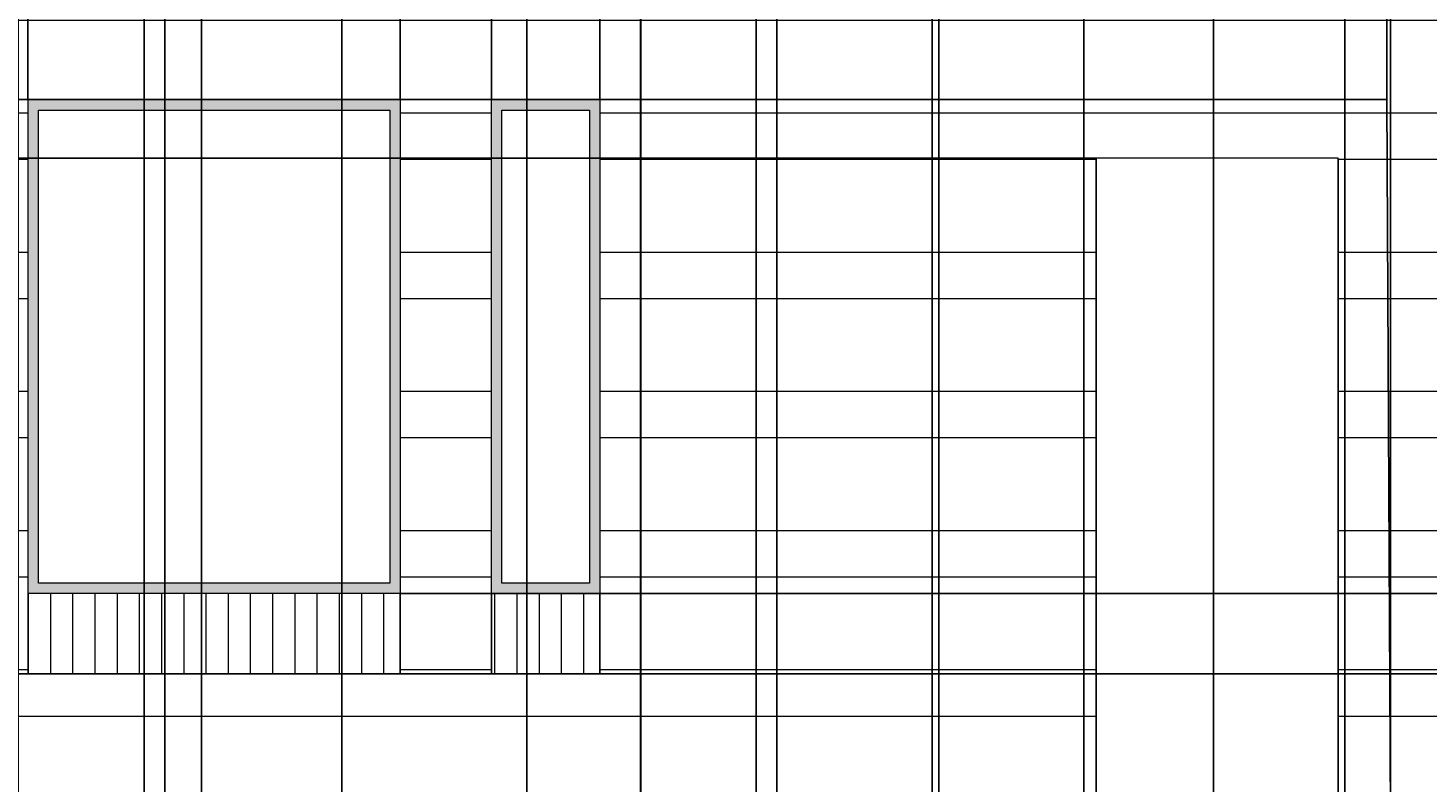
# Model space of a CAD drawing. Units: inches. Extents: x 241 to 943, y 109 to 1396.
# Tile 3 of 34: x 391 to 659, y 253 to 398. Entities that reach past the tile are written whole.
import ezdxf

# ---------------------------------------------------------------- set-up
doc = ezdxf.new("R2010")
doc.units = ezdxf.units.IN
doc.header["$MEASUREMENT"] = 0
for name, color, linetype, lineweight in [('A-ANNO-DIMS', 2, 'Continuous', 18), ('A-ELEV', 7, 'Continuous', 25), ('A-ELEV-SHAD', 9, 'Continuous', 13), ('A-GLAZ', 4, 'Continuous', 18), ('A-GLAZ-PATT', 18, 'Continuous', 13), ('A-WALL-PATT', 8, 'Continuous', 13)]:
    doc.layers.add(name, color=color, linetype=linetype, lineweight=lineweight)
doc.styles.get("Standard").update_dxf_attribs({"font": 'arial.ttf'})
doc.dimstyles.get("Standard").update_dxf_attribs({"dimtxt": 1.4375, "dimasz": 0.18, "dimexe": 0.18, "dimexo": 0.0625, "dimgap": 0.09, "dimtad": 0, "dimtih": 1, "dimtoh": 1, "dimdec": 4, "dimzin": 0, "dimdsep": 46, "dimlunit": 4, "dimtxsty": 'Standard', "dimcen": 0.09, "dimadec": 0, "dimazin": 0, "dimtfac": 1, "dimtdec": 4, "dimtofl": 0, "dimtmove": 0, "dimatfit": 3, "dimfxl": 1, "dimtolj": 1, "dimtzin": 0, "dimarcsym": 0})

# ---------------------------------------------------------------- blocks, each defined once
blk = doc.blocks.new('*D7')
at = {"layer": 'A-ANNO-DIMS', "color": 0, "lineweight": -2, "transparency": 16777216}
for p, q in [((508.24, 1336.12), (244.31, 1336.12)), ((244.49, 1335.94), (244.49, 753.25)), ((244.49, 168.92), (244.49, 751.6)), ((303.17, 168.74), (244.31, 168.74))]:
    blk.add_line(p, q, dxfattribs=at)
at = {"layer": 'A-ANNO-DIMS', "color": 0, "transparency": 16777216}
for points in [[(244.46, 1335.94), (244.52, 1335.94), (244.49, 1336.12)], [(244.46, 168.92), (244.52, 168.92), (244.49, 168.74)]]:
    blk.add_solid(points, dxfattribs=at)
at = {"layer": 'Defpoints', "color": 0, "transparency": 16777216}
for p in [(244.49, 1336.12), (508.31, 1336.12), (303.24, 168.74)]:
    blk.add_point(p, dxfattribs=at)
at = {"layer": 'A-ANNO-DIMS', "color": 0, "transparency": 16777216, "insert": (244.49, 752.43), "char_height": 1.438, "attachment_point": 5}
blk.add_mtext('\\A1;1167.4', dxfattribs=at)
blk = doc.blocks.new('*D9')
at = {"layer": 'A-ANNO-DIMS', "color": 0, "lineweight": -2, "transparency": 16777216}
for p, q in [((390.89, 384.24), (390.89, 1395.05)), ((391.07, 1394.87), (424.13, 1394.87)), ((461.93, 1394.87), (428.87, 1394.87)), ((462.11, 384.24), (462.11, 1395.05))]:
    blk.add_line(p, q, dxfattribs=at)
at = {"layer": 'A-ANNO-DIMS', "color": 0, "transparency": 16777216}
for points in [[(391.07, 1394.9), (391.07, 1394.84), (390.89, 1394.87)], [(461.93, 1394.9), (461.93, 1394.84), (462.11, 1394.87)]]:
    blk.add_solid(points, dxfattribs=at)
at = {"layer": 'Defpoints', "color": 0, "transparency": 16777216}
for p in [(462.11, 1394.87), (390.89, 384.18), (462.11, 384.18)]:
    blk.add_point(p, dxfattribs=at)
at = {"layer": 'A-ANNO-DIMS', "color": 0, "transparency": 16777216, "insert": (426.5, 1394.87), "char_height": 1.438, "attachment_point": 5}
blk.add_mtext('\\A1;71.21', dxfattribs=at)
blk = doc.blocks.new('*D10')
at = {"layer": 'A-ANNO-DIMS', "color": 0, "lineweight": -2, "transparency": 16777216}
for p, q in [((462.11, 384.24), (462.11, 1395.05)), ((462.29, 1394.87), (468.4, 1394.87)), ((479.42, 1394.87), (473.3, 1394.87)), ((479.6, 384.24), (479.6, 1395.05))]:
    blk.add_line(p, q, dxfattribs=at)
at = {"layer": 'A-ANNO-DIMS', "color": 0, "transparency": 16777216}
for points in [[(462.29, 1394.9), (462.29, 1394.84), (462.11, 1394.87)], [(479.42, 1394.9), (479.42, 1394.84), (479.6, 1394.87)]]:
    blk.add_solid(points, dxfattribs=at)
at = {"layer": 'Defpoints', "color": 0, "transparency": 16777216}
for p in [(479.6, 1394.87), (462.11, 384.18), (479.6, 384.18)]:
    blk.add_point(p, dxfattribs=at)
at = {"layer": 'A-ANNO-DIMS', "color": 0, "transparency": 16777216, "insert": (470.85, 1394.87), "char_height": 1.438, "attachment_point": 5}
blk.add_mtext('\\A1;17.49', dxfattribs=at)
blk = doc.blocks.new('*D11')
at = {"layer": 'A-ANNO-DIMS', "color": 0, "lineweight": -2, "transparency": 16777216}
for p, q in [((500.33, 384.24), (500.33, 1395.05)), ((500.51, 1394.87), (513.31, 1394.87)), ((530.05, 1394.87), (517.25, 1394.87)), ((530.23, 384.24), (530.23, 1395.05))]:
    blk.add_line(p, q, dxfattribs=at)
at = {"layer": 'A-ANNO-DIMS', "color": 0, "transparency": 16777216}
for points in [[(500.51, 1394.9), (500.51, 1394.84), (500.33, 1394.87)], [(530.05, 1394.9), (530.05, 1394.84), (530.23, 1394.87)]]:
    blk.add_solid(points, dxfattribs=at)
at = {"layer": 'Defpoints', "color": 0, "transparency": 16777216}
for p in [(530.23, 1394.87), (500.33, 384.18), (530.23, 384.18)]:
    blk.add_point(p, dxfattribs=at)
at = {"layer": 'A-ANNO-DIMS', "color": 0, "transparency": 16777216, "insert": (515.28, 1394.87), "char_height": 1.438, "attachment_point": 5}
blk.add_mtext('\\A1;29.9', dxfattribs=at)
blk = doc.blocks.new('*D12')
at = {"layer": 'A-ANNO-DIMS', "color": 0, "lineweight": -2, "transparency": 16777216}
for p, q in [((530.23, 384.24), (530.23, 1395.05)), ((530.41, 1394.87), (587.56, 1394.87)), ((650.73, 1394.87), (593.58, 1394.87)), ((650.91, 384.24), (650.91, 1395.05))]:
    blk.add_line(p, q, dxfattribs=at)
at = {"layer": 'A-ANNO-DIMS', "color": 0, "transparency": 16777216}
for points in [[(530.41, 1394.9), (530.41, 1394.84), (530.23, 1394.87)], [(650.73, 1394.9), (650.73, 1394.84), (650.91, 1394.87)]]:
    blk.add_solid(points, dxfattribs=at)
at = {"layer": 'Defpoints', "color": 0, "transparency": 16777216}
for p in [(650.91, 1394.87), (530.23, 384.18), (650.91, 384.18)]:
    blk.add_point(p, dxfattribs=at)
at = {"layer": 'A-ANNO-DIMS', "color": 0, "transparency": 16777216, "insert": (590.57, 1394.87), "char_height": 1.438, "attachment_point": 5}
blk.add_mtext('\\A1;120.68', dxfattribs=at)
blk = doc.blocks.new('*D13')
at = {"layer": 'A-ANNO-DIMS', "color": 0, "lineweight": -2, "transparency": 16777216}
for p, q in [((650.91, 384.24), (650.91, 1395.05)), ((651.09, 1394.87), (656.14, 1394.87)), ((667.21, 1394.87), (662.16, 1394.87)), ((667.39, 290.06), (667.39, 1395.05))]:
    blk.add_line(p, q, dxfattribs=at)
at = {"layer": 'A-ANNO-DIMS', "color": 0, "transparency": 16777216}
for points in [[(651.09, 1394.9), (651.09, 1394.84), (650.91, 1394.87)], [(667.21, 1394.9), (667.21, 1394.84), (667.39, 1394.87)]]:
    blk.add_solid(points, dxfattribs=at)
at = {"layer": 'Defpoints', "color": 0, "transparency": 16777216}
for p in [(667.39, 1394.87), (650.91, 384.18), (667.39, 290)]:
    blk.add_point(p, dxfattribs=at)
at = {"layer": 'A-ANNO-DIMS', "color": 0, "transparency": 16777216, "insert": (659.15, 1394.87), "char_height": 1.438, "attachment_point": 5}
blk.add_mtext('\\A1;16.486', dxfattribs=at)
blk = doc.blocks.new('*D16')
at = {"layer": 'A-ANNO-DIMS', "color": 0, "lineweight": -2, "transparency": 16777216}
for p, q in [((595.31, 372.88), (595.31, 109.81)), ((641.62, 372.88), (641.62, 109.81)), ((595.49, 109.99), (616.06, 109.99)), ((641.44, 109.99), (620.87, 109.99))]:
    blk.add_line(p, q, dxfattribs=at)
at = {"layer": 'A-ANNO-DIMS', "color": 0, "transparency": 16777216}
for points in [[(595.49, 110.02), (595.49, 109.96), (595.31, 109.99)], [(641.44, 110.02), (641.44, 109.96), (641.62, 109.99)]]:
    blk.add_solid(points, dxfattribs=at)
at = {"layer": 'Defpoints', "color": 0, "transparency": 16777216}
for p in [(595.31, 372.94), (641.62, 372.94), (641.62, 109.99)]:
    blk.add_point(p, dxfattribs=at)
at = {"layer": 'A-ANNO-DIMS', "color": 0, "transparency": 16777216, "insert": (618.47, 109.99), "char_height": 1.438, "attachment_point": 5}
blk.add_mtext('\\A1;46.31', dxfattribs=at)
blk = doc.blocks.new('*D29')
at = {"layer": 'A-ANNO-DIMS', "color": 0, "lineweight": -2, "transparency": 16777216}
for p, q in [((462.17, 289.69), (940.6, 289.69)), ((940.42, 289.51), (940.42, 282.85)), ((940.42, 274.53), (940.42, 281.2)), ((462.17, 274.35), (940.6, 274.35))]:
    blk.add_line(p, q, dxfattribs=at)
at = {"layer": 'A-ANNO-DIMS', "color": 0, "transparency": 16777216}
for points in [[(940.39, 289.51), (940.45, 289.51), (940.42, 289.69)], [(940.39, 274.53), (940.45, 274.53), (940.42, 274.35)]]:
    blk.add_solid(points, dxfattribs=at)
at = {"layer": 'Defpoints', "color": 0, "transparency": 16777216}
for p in [(462.11, 289.69), (940.42, 289.69), (462.11, 274.35)]:
    blk.add_point(p, dxfattribs=at)
at = {"layer": 'A-ANNO-DIMS', "color": 0, "transparency": 16777216, "insert": (940.42, 282.02), "char_height": 1.438, "attachment_point": 5}
blk.add_mtext('\\A1;15.343', dxfattribs=at)
blk = doc.blocks.new('*D41')
at = {"layer": 'A-ANNO-DIMS', "color": 0, "lineweight": -2, "transparency": 16777216}
for p, q in [((820.77, 400.83), (244.31, 400.83)), ((244.49, 400.65), (244.49, 317.65)), ((244.49, 233.01), (244.49, 316.01)), ((820.77, 232.83), (244.31, 232.83))]:
    blk.add_line(p, q, dxfattribs=at)
at = {"layer": 'A-ANNO-DIMS', "color": 0, "transparency": 16777216}
for points in [[(244.46, 400.65), (244.52, 400.65), (244.49, 400.83)], [(244.46, 233.01), (244.52, 233.01), (244.49, 232.83)]]:
    blk.add_solid(points, dxfattribs=at)
at = {"layer": 'Defpoints', "color": 0, "transparency": 16777216}
for p in [(244.49, 400.83), (820.84, 400.83), (820.84, 232.83)]:
    blk.add_point(p, dxfattribs=at)
at = {"layer": 'A-ANNO-DIMS', "color": 0, "transparency": 16777216, "insert": (244.49, 316.83), "char_height": 1.438, "attachment_point": 5}
blk.add_mtext('\\A1;168', dxfattribs=at)
blk = doc.blocks.new('*D51')
at = {"layer": 'A-ANNO-DIMS', "color": 0, "lineweight": -2, "transparency": 16777216}
for p, q in [((595.25, 372.94), (244.31, 372.94)), ((244.49, 372.76), (244.49, 310.39)), ((244.49, 246.38), (244.49, 308.74)), ((595.25, 246.2), (244.31, 246.2))]:
    blk.add_line(p, q, dxfattribs=at)
at = {"layer": 'A-ANNO-DIMS', "color": 0, "transparency": 16777216}
for points in [[(244.46, 372.76), (244.52, 372.76), (244.49, 372.94)], [(244.46, 246.38), (244.52, 246.38), (244.49, 246.2)]]:
    blk.add_solid(points, dxfattribs=at)
at = {"layer": 'Defpoints', "color": 0, "transparency": 16777216}
for p in [(244.49, 372.94), (595.31, 372.94), (595.31, 246.2)]:
    blk.add_point(p, dxfattribs=at)
at = {"layer": 'A-ANNO-DIMS', "color": 0, "transparency": 16777216, "insert": (244.49, 309.57), "char_height": 1.438, "attachment_point": 5}
blk.add_mtext('\\A1;126.74', dxfattribs=at)
blk = doc.blocks.new('*D52')
at = {"layer": 'A-ANNO-DIMS', "color": 0, "lineweight": -2, "transparency": 16777216}
for p, q in [((530.17, 384.18), (244.31, 384.18)), ((244.49, 384), (244.49, 315.83)), ((244.49, 246.02), (244.49, 314.18)), ((530.17, 245.84), (244.31, 245.84))]:
    blk.add_line(p, q, dxfattribs=at)
at = {"layer": 'A-ANNO-DIMS', "color": 0, "transparency": 16777216}
for points in [[(244.46, 384), (244.52, 384), (244.49, 384.18)], [(244.46, 246.02), (244.52, 246.02), (244.49, 245.84)]]:
    blk.add_solid(points, dxfattribs=at)
at = {"layer": 'Defpoints', "color": 0, "transparency": 16777216}
for p in [(244.49, 384.18), (530.23, 384.18), (530.23, 245.84)]:
    blk.add_point(p, dxfattribs=at)
at = {"layer": 'A-ANNO-DIMS', "color": 0, "transparency": 16777216, "insert": (244.49, 315.01), "char_height": 1.438, "attachment_point": 5}
blk.add_mtext('\\A1;138.34', dxfattribs=at)
blk = doc.blocks.new('*D79')
at = {"layer": 'A-ANNO-DIMS', "color": 0, "lineweight": -2, "transparency": 16777216}
for p, q in [((479.6, 384.24), (479.6, 1395.05)), ((479.78, 1394.87), (486.88, 1394.87)), ((500.15, 1394.87), (493.05, 1394.87)), ((500.33, 384.24), (500.33, 1395.05))]:
    blk.add_line(p, q, dxfattribs=at)
at = {"layer": 'A-ANNO-DIMS', "color": 0, "transparency": 16777216}
for points in [[(479.78, 1394.9), (479.78, 1394.84), (479.6, 1394.87)], [(500.15, 1394.9), (500.15, 1394.84), (500.33, 1394.87)]]:
    blk.add_solid(points, dxfattribs=at)
at = {"layer": 'Defpoints', "color": 0, "transparency": 16777216}
for p in [(500.33, 1394.87), (479.6, 384.18), (500.33, 384.18)]:
    blk.add_point(p, dxfattribs=at)
at = {"layer": 'A-ANNO-DIMS', "color": 0, "transparency": 16777216, "insert": (489.96, 1394.87), "char_height": 1.438, "attachment_point": 5}
blk.add_mtext('\\A1;20.736', dxfattribs=at)
blk = doc.blocks.new('*D80')
at = {"layer": 'A-ANNO-DIMS', "color": 0, "lineweight": -2, "transparency": 16777216}
for p, q in [((530.23, 384.12), (530.23, 109.81)), ((595.31, 372.88), (595.31, 109.81)), ((530.41, 109.99), (560.25, 109.99)), ((595.13, 109.99), (565.29, 109.99))]:
    blk.add_line(p, q, dxfattribs=at)
at = {"layer": 'A-ANNO-DIMS', "color": 0, "transparency": 16777216}
for points in [[(530.41, 110.02), (530.41, 109.96), (530.23, 109.99)], [(595.13, 110.02), (595.13, 109.96), (595.31, 109.99)]]:
    blk.add_solid(points, dxfattribs=at)
at = {"layer": 'Defpoints', "color": 0, "transparency": 16777216}
for p in [(530.23, 384.18), (595.31, 372.94), (595.31, 109.99)]:
    blk.add_point(p, dxfattribs=at)
at = {"layer": 'A-ANNO-DIMS', "color": 0, "transparency": 16777216, "insert": (562.77, 109.99), "char_height": 1.438, "attachment_point": 5}
blk.add_mtext('\\A1;65.08', dxfattribs=at)
blk = doc.blocks.new('*D81')
at = {"layer": 'A-ANNO-DIMS', "color": 0, "lineweight": -2, "transparency": 16777216}
for p, q in [((462.04, 274.35), (244.31, 274.35)), ((244.49, 274.17), (244.49, 260.92)), ((244.49, 246.02), (244.49, 259.27)), ((530.17, 245.84), (244.31, 245.84))]:
    blk.add_line(p, q, dxfattribs=at)
at = {"layer": 'A-ANNO-DIMS', "color": 0, "transparency": 16777216}
for points in [[(244.46, 274.17), (244.52, 274.17), (244.49, 274.35)], [(244.46, 246.02), (244.52, 246.02), (244.49, 245.84)]]:
    blk.add_solid(points, dxfattribs=at)
at = {"layer": 'Defpoints', "color": 0, "transparency": 16777216}
for p in [(244.49, 274.35), (462.11, 274.35), (530.23, 245.84)]:
    blk.add_point(p, dxfattribs=at)
at = {"layer": 'A-ANNO-DIMS', "color": 0, "transparency": 16777216, "insert": (244.49, 260.09), "char_height": 1.438, "attachment_point": 5}
blk.add_mtext('\\A1;28.51', dxfattribs=at)
blk = doc.blocks.new('*D99')
at = {"layer": 'A-ANNO-DIMS', "color": 0, "lineweight": -2, "transparency": 16777216}
for p, q in [((417.09, 181.71), (417.09, 1395.05)), ((417.27, 1394.87), (539.16, 1394.87)), ((667.21, 1394.87), (545.33, 1394.87)), ((667.39, 214.58), (667.39, 1395.05))]:
    blk.add_line(p, q, dxfattribs=at)
at = {"layer": 'A-ANNO-DIMS', "color": 0, "transparency": 16777216}
for points in [[(417.27, 1394.9), (417.27, 1394.84), (417.09, 1394.87)], [(667.21, 1394.9), (667.21, 1394.84), (667.39, 1394.87)]]:
    blk.add_solid(points, dxfattribs=at)
at = {"layer": 'Defpoints', "color": 0, "transparency": 16777216}
for p in [(667.39, 1394.87), (667.39, 214.52), (417.09, 181.65)]:
    blk.add_point(p, dxfattribs=at)
at = {"layer": 'A-ANNO-DIMS', "color": 0, "transparency": 16777216, "insert": (542.24, 1394.87), "char_height": 1.438, "attachment_point": 5}
blk.add_mtext('\\A1;250.30', dxfattribs=at)
blk = doc.blocks.new('*D119')
at = {"layer": 'A-ANNO-DIMS', "color": 0, "lineweight": -2, "transparency": 16777216}
for p, q in [((617.76, 734.79), (617.76, 109.81)), ((642.92, 734.79), (642.92, 109.81)), ((617.94, 109.99), (627.81, 109.99)), ((642.74, 109.99), (632.87, 109.99))]:
    blk.add_line(p, q, dxfattribs=at)
at = {"layer": 'A-ANNO-DIMS', "color": 0, "transparency": 16777216}
for points in [[(617.94, 110.02), (617.94, 109.96), (617.76, 109.99)], [(642.74, 110.02), (642.74, 109.96), (642.92, 109.99)]]:
    blk.add_solid(points, dxfattribs=at)
at = {"layer": 'Defpoints', "color": 0, "transparency": 16777216}
for p in [(617.76, 734.85), (642.92, 734.85), (642.92, 109.99)]:
    blk.add_point(p, dxfattribs=at)
at = {"layer": 'A-ANNO-DIMS', "color": 0, "transparency": 16777216, "insert": (630.34, 109.99), "char_height": 1.438, "attachment_point": 5}
blk.add_mtext('\\A1;25.16', dxfattribs=at)
blk = doc.blocks.new('*D120')
at = {"layer": 'A-ANNO-DIMS', "color": 0, "lineweight": -2, "transparency": 16777216}
for p, q in [((642.92, 734.79), (642.92, 109.81)), ((678.27, 734.79), (678.27, 109.81)), ((643.1, 109.99), (658.07, 109.99)), ((678.09, 109.99), (663.11, 109.99))]:
    blk.add_line(p, q, dxfattribs=at)
at = {"layer": 'A-ANNO-DIMS', "color": 0, "transparency": 16777216}
for points in [[(643.1, 110.02), (643.1, 109.96), (642.92, 109.99)], [(678.09, 110.02), (678.09, 109.96), (678.27, 109.99)]]:
    blk.add_solid(points, dxfattribs=at)
at = {"layer": 'Defpoints', "color": 0, "transparency": 16777216}
for p in [(642.92, 734.85), (678.27, 734.85), (678.27, 109.99)]:
    blk.add_point(p, dxfattribs=at)
at = {"layer": 'A-ANNO-DIMS', "color": 0, "transparency": 16777216, "insert": (660.59, 109.99), "char_height": 1.438, "attachment_point": 5}
blk.add_mtext('\\A1;35.35', dxfattribs=at)
blk = doc.blocks.new('*D126')
at = {"layer": 'A-ANNO-DIMS', "color": 0, "lineweight": -2, "transparency": 16777216}
for p, q in [((450.93, 651.27), (450.93, 109.81)), ((424.11, 628.34), (424.11, 109.81)), ((424.29, 109.99), (434.43, 109.99)), ((450.75, 109.99), (440.6, 109.99))]:
    blk.add_line(p, q, dxfattribs=at)
at = {"layer": 'A-ANNO-DIMS', "color": 0, "transparency": 16777216}
for points in [[(424.29, 110.02), (424.29, 109.96), (424.11, 109.99)], [(450.75, 110.02), (450.75, 109.96), (450.93, 109.99)]]:
    blk.add_solid(points, dxfattribs=at)
at = {"layer": 'Defpoints', "color": 0, "transparency": 16777216}
for p in [(450.93, 651.34), (424.11, 628.4), (450.93, 109.99)]:
    blk.add_point(p, dxfattribs=at)
at = {"layer": 'A-ANNO-DIMS', "color": 0, "transparency": 16777216, "insert": (437.52, 109.99), "char_height": 1.438, "attachment_point": 5}
blk.add_mtext('\\A1;26.817', dxfattribs=at)
blk = doc.blocks.new('*D127')
at = {"layer": 'A-ANNO-DIMS', "color": 0, "lineweight": -2, "transparency": 16777216}
for p, q in [((450.93, 651.27), (450.93, 109.81)), ((508.19, 630.34), (508.19, 109.81)), ((451.11, 109.99), (477.04, 109.99)), ((508.01, 109.99), (482.07, 109.99))]:
    blk.add_line(p, q, dxfattribs=at)
at = {"layer": 'A-ANNO-DIMS', "color": 0, "transparency": 16777216}
for points in [[(451.11, 110.02), (451.11, 109.96), (450.93, 109.99)], [(508.01, 110.02), (508.01, 109.96), (508.19, 109.99)]]:
    blk.add_solid(points, dxfattribs=at)
at = {"layer": 'Defpoints', "color": 0, "transparency": 16777216}
for p in [(450.93, 651.34), (508.19, 630.4), (508.19, 109.99)]:
    blk.add_point(p, dxfattribs=at)
at = {"layer": 'A-ANNO-DIMS', "color": 0, "transparency": 16777216, "insert": (479.56, 109.99), "char_height": 1.438, "attachment_point": 5}
blk.add_mtext('\\A1;57.26', dxfattribs=at)
blk = doc.blocks.new('*D128')
at = {"layer": 'A-ANNO-DIMS', "color": 0, "lineweight": -2, "transparency": 16777216}
for p, q in [((534.18, 651.27), (534.18, 109.81)), ((508.19, 630.34), (508.19, 109.81)), ((508.37, 109.99), (518.1, 109.99)), ((534, 109.99), (524.27, 109.99))]:
    blk.add_line(p, q, dxfattribs=at)
at = {"layer": 'A-ANNO-DIMS', "color": 0, "transparency": 16777216}
for points in [[(508.37, 110.02), (508.37, 109.96), (508.19, 109.99)], [(534, 110.02), (534, 109.96), (534.18, 109.99)]]:
    blk.add_solid(points, dxfattribs=at)
at = {"layer": 'Defpoints', "color": 0, "transparency": 16777216}
for p in [(534.18, 651.34), (508.19, 630.4), (534.18, 109.99)]:
    blk.add_point(p, dxfattribs=at)
at = {"layer": 'A-ANNO-DIMS', "color": 0, "transparency": 16777216, "insert": (521.18, 109.99), "char_height": 1.438, "attachment_point": 5}
blk.add_mtext('\\A1;25.987', dxfattribs=at)
blk = doc.blocks.new('*D129')
at = {"layer": 'A-ANNO-DIMS', "color": 0, "lineweight": -2, "transparency": 16777216}
for p, q in [((534.18, 651.27), (534.18, 109.81)), ((563.93, 651.27), (563.93, 109.81)), ((534.36, 109.99), (546.52, 109.99)), ((563.75, 109.99), (551.59, 109.99))]:
    blk.add_line(p, q, dxfattribs=at)
at = {"layer": 'A-ANNO-DIMS', "color": 0, "transparency": 16777216}
for points in [[(534.36, 110.02), (534.36, 109.96), (534.18, 109.99)], [(563.75, 110.02), (563.75, 109.96), (563.93, 109.99)]]:
    blk.add_solid(points, dxfattribs=at)
at = {"layer": 'Defpoints', "color": 0, "transparency": 16777216}
for p in [(534.18, 651.34), (563.93, 651.34), (563.93, 109.99)]:
    blk.add_point(p, dxfattribs=at)
at = {"layer": 'A-ANNO-DIMS', "color": 0, "transparency": 16777216, "insert": (549.05, 109.99), "char_height": 1.438, "attachment_point": 5}
blk.add_mtext('\\A1;29.75', dxfattribs=at)
blk = doc.blocks.new('*D130')
at = {"layer": 'A-ANNO-DIMS', "color": 0, "lineweight": -2, "transparency": 16777216}
for p, q in [((563.93, 651.27), (563.93, 109.81)), ((592.95, 628.34), (592.95, 109.81)), ((564.11, 109.99), (575.35, 109.99)), ((592.77, 109.99), (581.53, 109.99))]:
    blk.add_line(p, q, dxfattribs=at)
at = {"layer": 'A-ANNO-DIMS', "color": 0, "transparency": 16777216}
for points in [[(564.11, 110.02), (564.11, 109.96), (563.93, 109.99)], [(592.77, 110.02), (592.77, 109.96), (592.95, 109.99)]]:
    blk.add_solid(points, dxfattribs=at)
at = {"layer": 'Defpoints', "color": 0, "transparency": 16777216}
for p in [(563.93, 651.34), (592.95, 628.4), (592.95, 109.99)]:
    blk.add_point(p, dxfattribs=at)
at = {"layer": 'A-ANNO-DIMS', "color": 0, "transparency": 16777216, "insert": (578.44, 109.99), "char_height": 1.438, "attachment_point": 5}
blk.add_mtext('\\A1;29.025', dxfattribs=at)
blk = doc.blocks.new('*D132')
at = {"layer": 'A-ANNO-DIMS', "color": 0, "lineweight": -2, "transparency": 16777216}
for p, q in [((676.87, 628.34), (676.87, 109.81)), ((617.76, 626.34), (617.76, 109.81)), ((617.94, 109.99), (644.94, 109.99)), ((676.69, 109.99), (649.69, 109.99))]:
    blk.add_line(p, q, dxfattribs=at)
at = {"layer": 'A-ANNO-DIMS', "color": 0, "transparency": 16777216}
for points in [[(617.94, 110.02), (617.94, 109.96), (617.76, 109.99)], [(676.69, 110.02), (676.69, 109.96), (676.87, 109.99)]]:
    blk.add_solid(points, dxfattribs=at)
at = {"layer": 'Defpoints', "color": 0, "transparency": 16777216}
for p in [(676.87, 628.4), (617.76, 626.4), (676.87, 109.99)]:
    blk.add_point(p, dxfattribs=at)
at = {"layer": 'A-ANNO-DIMS', "color": 0, "transparency": 16777216, "insert": (647.31, 109.99), "char_height": 1.438, "attachment_point": 5}
blk.add_mtext('\\A1;59.11', dxfattribs=at)
blk = doc.blocks.new('*D136')
at = {"layer": 'A-ANNO-DIMS', "color": 0, "lineweight": -2, "transparency": 16777216}
for p, q in [((450.93, 519.31), (450.93, 109.81)), ((424.11, 496.38), (424.11, 109.81)), ((424.29, 109.99), (434.43, 109.99)), ((450.75, 109.99), (440.6, 109.99))]:
    blk.add_line(p, q, dxfattribs=at)
at = {"layer": 'A-ANNO-DIMS', "color": 0, "transparency": 16777216}
for points in [[(424.29, 110.02), (424.29, 109.96), (424.11, 109.99)], [(450.75, 110.02), (450.75, 109.96), (450.93, 109.99)]]:
    blk.add_solid(points, dxfattribs=at)
at = {"layer": 'Defpoints', "color": 0, "transparency": 16777216}
for p in [(450.93, 519.38), (424.11, 496.44), (450.93, 109.99)]:
    blk.add_point(p, dxfattribs=at)
at = {"layer": 'A-ANNO-DIMS', "color": 0, "transparency": 16777216, "insert": (437.52, 109.99), "char_height": 1.438, "attachment_point": 5}
blk.add_mtext('\\A1;26.817', dxfattribs=at)
blk = doc.blocks.new('*D137')
at = {"layer": 'A-ANNO-DIMS', "color": 0, "lineweight": -2, "transparency": 16777216}
for p, q in [((450.93, 519.31), (450.93, 109.81)), ((508.08, 508.84), (508.08, 109.81)), ((451.11, 109.99), (476.98, 109.99)), ((507.9, 109.99), (482.02, 109.99))]:
    blk.add_line(p, q, dxfattribs=at)
at = {"layer": 'A-ANNO-DIMS', "color": 0, "transparency": 16777216}
for points in [[(451.11, 110.02), (451.11, 109.96), (450.93, 109.99)], [(507.9, 110.02), (507.9, 109.96), (508.08, 109.99)]]:
    blk.add_solid(points, dxfattribs=at)
at = {"layer": 'Defpoints', "color": 0, "transparency": 16777216}
for p in [(450.93, 519.38), (508.08, 508.91), (508.08, 109.99)]:
    blk.add_point(p, dxfattribs=at)
at = {"layer": 'A-ANNO-DIMS', "color": 0, "transparency": 16777216, "insert": (479.5, 109.99), "char_height": 1.438, "attachment_point": 5}
blk.add_mtext('\\A1;57.15', dxfattribs=at)
blk = doc.blocks.new('*D138')
at = {"layer": 'A-ANNO-DIMS', "color": 0, "lineweight": -2, "transparency": 16777216}
for p, q in [((508.08, 508.84), (508.08, 109.81)), ((534.18, 508.84), (534.18, 109.81)), ((508.26, 109.99), (518.6, 109.99)), ((534, 109.99), (523.65, 109.99))]:
    blk.add_line(p, q, dxfattribs=at)
at = {"layer": 'A-ANNO-DIMS', "color": 0, "transparency": 16777216}
for points in [[(508.26, 110.02), (508.26, 109.96), (508.08, 109.99)], [(534, 110.02), (534, 109.96), (534.18, 109.99)]]:
    blk.add_solid(points, dxfattribs=at)
at = {"layer": 'Defpoints', "color": 0, "transparency": 16777216}
for p in [(508.08, 508.91), (534.18, 508.91), (534.18, 109.99)]:
    blk.add_point(p, dxfattribs=at)
at = {"layer": 'A-ANNO-DIMS', "color": 0, "transparency": 16777216, "insert": (521.13, 109.99), "char_height": 1.438, "attachment_point": 5}
blk.add_mtext('\\A1;26.10', dxfattribs=at)
blk = doc.blocks.new('*D139')
at = {"layer": 'A-ANNO-DIMS', "color": 0, "lineweight": -2, "transparency": 16777216}
for p, q in [((534.18, 508.84), (534.18, 109.81)), ((565.2, 496.38), (565.2, 109.81)), ((534.36, 109.99), (546.61, 109.99)), ((565.02, 109.99), (552.77, 109.99))]:
    blk.add_line(p, q, dxfattribs=at)
at = {"layer": 'A-ANNO-DIMS', "color": 0, "transparency": 16777216}
for points in [[(534.36, 110.02), (534.36, 109.96), (534.18, 109.99)], [(565.02, 110.02), (565.02, 109.96), (565.2, 109.99)]]:
    blk.add_solid(points, dxfattribs=at)
at = {"layer": 'Defpoints', "color": 0, "transparency": 16777216}
for p in [(534.18, 508.91), (565.2, 496.44), (565.2, 109.99)]:
    blk.add_point(p, dxfattribs=at)
at = {"layer": 'A-ANNO-DIMS', "color": 0, "transparency": 16777216, "insert": (549.69, 109.99), "char_height": 1.438, "attachment_point": 5}
blk.add_mtext('\\A1;31.025', dxfattribs=at)
blk = doc.blocks.new('*D142')
at = {"layer": 'A-ANNO-DIMS', "color": 0, "lineweight": -2, "transparency": 16777216}
for p, q in [((689.79, 498.38), (689.79, 109.81)), ((651.6, 496.38), (651.6, 109.81)), ((651.78, 109.99), (668.18, 109.99)), ((689.61, 109.99), (673.21, 109.99))]:
    blk.add_line(p, q, dxfattribs=at)
at = {"layer": 'A-ANNO-DIMS', "color": 0, "transparency": 16777216}
for points in [[(651.78, 110.02), (651.78, 109.96), (651.6, 109.99)], [(689.61, 110.02), (689.61, 109.96), (689.79, 109.99)]]:
    blk.add_solid(points, dxfattribs=at)
at = {"layer": 'Defpoints', "color": 0, "transparency": 16777216}
for p in [(689.79, 498.44), (651.6, 496.44), (689.79, 109.99)]:
    blk.add_point(p, dxfattribs=at)
at = {"layer": 'A-ANNO-DIMS', "color": 0, "transparency": 16777216, "insert": (670.7, 109.99), "char_height": 1.438, "attachment_point": 5}
blk.add_mtext('\\A1;38.20', dxfattribs=at)
blk = doc.blocks.new('*D147')
at = {"layer": 'A-ANNO-DIMS', "color": 0, "lineweight": -2, "transparency": 16777216}
for p, q in [((389.04, 734.79), (389.04, 109.81)), ((413.12, 734.79), (413.12, 109.81)), ((389.22, 109.99), (398, 109.99)), ((412.94, 109.99), (404.17, 109.99))]:
    blk.add_line(p, q, dxfattribs=at)
at = {"layer": 'A-ANNO-DIMS', "color": 0, "transparency": 16777216}
for points in [[(389.22, 110.02), (389.22, 109.96), (389.04, 109.99)], [(412.94, 110.02), (412.94, 109.96), (413.12, 109.99)]]:
    blk.add_solid(points, dxfattribs=at)
at = {"layer": 'Defpoints', "color": 0, "transparency": 16777216}
for p in [(389.04, 734.85), (413.12, 734.85), (413.12, 109.99)]:
    blk.add_point(p, dxfattribs=at)
at = {"layer": 'A-ANNO-DIMS', "color": 0, "transparency": 16777216, "insert": (401.08, 109.99), "char_height": 1.438, "attachment_point": 5}
blk.add_mtext('\\A1;24.076', dxfattribs=at)
blk = doc.blocks.new('*D148')
at = {"layer": 'A-ANNO-DIMS', "color": 0, "lineweight": -2, "transparency": 16777216}
for p, q in [((413.12, 734.79), (413.12, 109.81)), ((486.34, 734.79), (486.34, 109.81)), ((413.3, 109.99), (447.23, 109.99)), ((486.16, 109.99), (452.23, 109.99))]:
    blk.add_line(p, q, dxfattribs=at)
at = {"layer": 'A-ANNO-DIMS', "color": 0, "transparency": 16777216}
for points in [[(413.3, 110.02), (413.3, 109.96), (413.12, 109.99)], [(486.16, 110.02), (486.16, 109.96), (486.34, 109.99)]]:
    blk.add_solid(points, dxfattribs=at)
at = {"layer": 'Defpoints', "color": 0, "transparency": 16777216}
for p in [(413.12, 734.85), (486.34, 734.85), (486.34, 109.99)]:
    blk.add_point(p, dxfattribs=at)
at = {"layer": 'A-ANNO-DIMS', "color": 0, "transparency": 16777216, "insert": (449.73, 109.99), "char_height": 1.438, "attachment_point": 5}
blk.add_mtext('\\A1;73.22', dxfattribs=at)

msp = doc.modelspace()

# ---------------------------------------------------------------- hatches: boundary and pattern name
at = {"layer": 'A-ELEV-SHAD'}
h = msp.add_hatch(color=256, dxfattribs=at)
h.dxf.hatch_style = 1
h.paths.add_polyline_path([(748.3325, 566.8295), (746.3325, 566.8295), (746.3325, 498.4395), (748.3325, 498.4395)])
h.paths.add_polyline_path([(746.3325, 524.3723), (691.794, 524.3723), (691.794, 522.3723), (746.3325, 522.3723)])
h.paths.add_polyline_path([(691.794, 566.8295), (689.794, 566.8295), (689.794, 498.4395), (691.794, 498.4395)])
h.paths.add_polyline_path([(790.691, 542.7994), (748.3325, 542.7994), (748.3325, 540.7994), (790.691, 540.7994)])
h.paths.add_polyline_path([(500.3323, 384.1784), (479.596, 384.1784), (479.596, 289.6933), (500.3323, 289.6933)])
h.paths.add_polyline_path([(481.596, 291.6933), (481.596, 382.1784), (498.3323, 382.1784), (498.3323, 291.6933)], flags=16)
h.paths.add_polyline_path([(462.1074, 384.1784), (390.895, 384.1784), (390.895, 289.6933), (462.1074, 289.6933)])
h.paths.add_polyline_path([(392.895, 291.6933), (392.895, 382.1784), (460.1074, 382.1784), (460.1074, 291.6933)], flags=16)
h.paths.add_polyline_path([(794.0275, 289.9984), (667.3935, 289.9984), (667.3935, 214.5189), (794.0275, 214.5189)])
h.paths.add_polyline_path([(792.0275, 287.9984), (792.0275, 216.5189), (669.3935, 216.5189), (669.3935, 287.9984)], flags=16)
h.paths.add_polyline_path([(508.0803, 525.3816), (506.0803, 525.3816), (506.0803, 521.3754), (452.9259, 521.3754), (452.9259, 525.3816), (450.9259, 525.3816), (450.9259, 519.3754), (508.0803, 519.3754)], flags=0)
h.paths.add_polyline_path([(508.0803, 566.8295), (450.9259, 566.8295), (450.9259, 527.3816), (452.9259, 527.3816), (452.9259, 564.8295), (506.0803, 564.8295), (506.0803, 527.3816), (508.0803, 527.3816)], flags=0)
h.paths.add_polyline_path([(537.4269, 566.8295), (534.1778, 566.8295), (534.1778, 527.3816), (537.4269, 527.3816)], flags=0)
h.paths.add_polyline_path([(537.4269, 525.3816), (534.1778, 525.3816), (534.1778, 508.9074), (537.4269, 508.9074)], flags=0)
h.paths.add_polyline_path([(565.2023, 568.8295), (424.1086, 568.8295), (424.1086, 496.4395), (565.2023, 496.4395)])
h.paths.add_polyline_path([(563.2023, 508.9074), (563.2023, 498.4395), (426.1086, 498.4395), (426.1086, 566.8295), (563.2023, 566.8295)], flags=16)
h.paths.add_polyline_path([(508.0803, 508.9074), (508.0803, 519.3754), (450.9259, 519.3754), (450.9259, 525.3816), (445.5808, 525.3816, -1), (445.5808, 527.3816), (450.9259, 527.3816), (450.9259, 566.8295), (508.0803, 566.8295), (537.4269, 566.8295), (537.4269, 508.9074)], flags=0)
h.paths.add_polyline_path([(506.0803, 521.3754), (452.9259, 521.3754), (452.9259, 564.8295), (506.0803, 564.8295)], flags=0)
at = {"layer": 'A-GLAZ-PATT'}
h = msp.add_hatch(dxfattribs=at)
h.set_pattern_fill('ANSI31', color=256, scale=34, angle=45)
h.paths.add_polyline_path([(486.3418, 786.9154), (413.1187, 786.9154), (413.1187, 761.2284), (486.3418, 761.2284)])
h.paths.add_polyline_path([(486.3418, 954.9154), (413.1187, 954.9154), (413.1187, 929.2284), (486.3418, 929.2284)])
h.paths.add_polyline_path([(462.1074, 289.6933), (390.895, 289.6933), (390.895, 277.4626), (390.895, 274.3507), (462.1074, 274.3507), (462.1074, 277.4626)])
h.paths.add_polyline_path([(500.3323, 289.6933), (479.596, 289.6933), (479.596, 274.3507), (500.3323, 274.3507)])
h.paths.add_polyline_path([(450.9259, 566.8295), (426.1086, 566.8295), (426.1086, 498.4395), (446.4348, 498.4395), (446.4348, 519.3754), (450.9259, 519.3754), (450.9259, 525.3816), (445.5808, 525.3816, -1), (445.5808, 527.3816), (450.9259, 527.3816)])
h.paths.add_polyline_path([(563.2023, 508.9074), (534.1778, 508.9074), (508.1906, 508.9074), (508.1906, 498.4395), (563.2023, 498.4395)])
h.paths.add_polyline_path([(747.6328, 700.7912), (712.0171, 700.7912), (712.0171, 628.4013), (747.6328, 628.4013)])
h.paths.add_polyline_path([(446.4348, 643.7483), (426.1086, 643.7483), (426.1086, 630.4013), (446.4348, 630.4013)])
h.paths.add_polyline_path([(564.8076, 841.5382), (553.5166, 841.5382), (508.3064, 841.5382), (508.3064, 782.5808), (564.8076, 782.5808)])
h.paths.add_polyline_path([(564.8076, 780.5808), (508.3064, 780.5808), (508.3064, 773.4916), (564.8076, 773.4916)])
h.paths.add_polyline_path([(792.691, 762.5799), (759.6248, 762.5799), (759.6248, 736.9235), (759.6248, 734.8538), (792.691, 734.8538)])
h.paths.add_polyline_path([(564.8076, 1009.5382), (553.5166, 1009.5382), (508.3064, 1009.5382), (508.3064, 950.5808), (562.3033, 950.5808, -1), (562.3033, 948.5808), (508.3064, 948.5808), (508.3064, 941.4916), (564.8076, 941.4916)])
h.paths.add_polyline_path([(486.3418, 1122.9154), (413.1187, 1122.9154), (413.1187, 1097.2284), (486.3418, 1097.2284)])
at = {"layer": 'A-WALL-PATT'}
h = msp.add_hatch(dxfattribs=at)
h.set_pattern_fill('ANSI32', color=256, scale=71, angle=135)
h.paths.add_polyline_path([(820.8374, 568.8295), (792.691, 568.8295), (792.691, 496.4395), (651.5974, 496.4395), (651.5974, 568.8295), (617.7594, 568.8295), (618.9643, 400.8295), (417.0913, 400.8295), (377.0391, 400.8295), (377.0391, 398.8538), (377.0391, 396.8782), (377.0391, 228.8782), (377.0391, 177.6977), (416.5078, 181.5724), (417.0913, 181.649), (530.2303, 196.5065), (530.2303, 384.1784), (650.907, 384.1784), (651.7861, 212.4693), (667.3935, 214.5189), (667.3935, 289.9984), (794.0275, 289.9984), (794.0275, 232.8295), (820.8374, 232.8295), (820.8374, 400.8295)])
h.paths.add_polyline_path([(500.3323, 384.1784), (500.3323, 289.6933), (500.3323, 274.3507), (479.596, 274.3507), (479.596, 289.6933), (479.596, 384.1784)], flags=16)
h.paths.add_polyline_path([(498.3323, 382.1784), (498.3323, 291.6933), (481.596, 291.6933), (481.596, 382.1784)], flags=0)
h.paths.add_polyline_path([(462.1074, 384.1784), (462.1074, 289.6933), (462.1074, 277.4626), (462.1074, 274.3507), (390.895, 274.3507), (390.895, 277.4626), (390.895, 289.6933), (390.895, 384.1784)], flags=16)
h.paths.add_polyline_path([(460.1074, 382.1784), (460.1074, 291.6933), (392.895, 291.6933), (392.895, 382.1784)], flags=0)
h.paths.add_polyline_path([(595.3136, 372.9401), (641.6196, 372.9401), (641.6196, 246.4081), (651.6121, 246.4593), (650.907, 384.1784), (530.2303, 384.1784), (530.2303, 245.8378), (595.3136, 246.1711)], flags=17)

# ---------------------------------------------------------------- linework, layer by layer
at = {"layer": 'A-ELEV'}
for p, q in [((530.2303, 196.5065), (530.2303, 384.1784)), ((530.2303, 384.1784), (650.907, 384.1784)), ((650.907, 384.1784), (651.7861, 212.4693)), ((390.895, 289.6933), (390.895, 277.4626)), ((462.1074, 277.4626), (462.1074, 289.6933)), ((479.596, 289.6933), (479.596, 274.3507)), ((500.3323, 274.3507), (500.3323, 289.6933)), ((390.895, 277.4626), (390.895, 274.3507)), ((462.1074, 277.4626), (462.1074, 274.3507)), ((390.895, 274.3507), (462.1074, 274.3507)), ((479.596, 274.3507), (500.3323, 274.3507))]:
    msp.add_line(p, q, dxfattribs=at)
at = {"layer": 'A-GLAZ'}
for points in [[(390.895, 384.1784), (462.1074, 384.1784), (462.1074, 289.6933), (390.895, 289.6933)], [(479.596, 384.1784), (500.3323, 384.1784), (500.3323, 289.6933), (479.596, 289.6933)], [(392.895, 382.1784), (460.1074, 382.1784), (460.1074, 291.6933), (392.895, 291.6933)], [(481.596, 382.1784), (498.3323, 382.1784), (498.3323, 291.6933), (481.596, 291.6933)], [(595.3136, 246.1966), (641.6196, 246.1966), (641.6196, 372.9401), (595.3136, 372.9401)]]:
    msp.add_lwpolyline(points, close=True, dxfattribs=at)

# ---------------------------------------------------------------- dimensions: what is measured, and where the dimension line sits
at = {"layer": 'A-ANNO-DIMS'}
for base, p1, p2, override, picture, middle in [((462.1074, 1394.8654), (390.895, 384.1784), (462.1074, 384.1784), {"dimdec": 2, "dimlfac": 1, "dimrnd": 0, "dimzin": 0, "dimdsep": 46, "dimlunit": 2}, '*D9', (426.5012, 1394.8654)), ((667.3935, 1394.8654), (417.0913, 181.649), (667.3935, 214.5189), {"dimdec": 2, "dimlfac": 1, "dimrnd": 0, "dimzin": 0, "dimdsep": 46, "dimlunit": 2}, '*D99', (542.2424, 1394.8654)), ((479.596, 1394.8654), (462.1074, 384.1784), (479.596, 384.1784), {"dimdec": 2, "dimlfac": 1, "dimrnd": 0, "dimzin": 0, "dimdsep": 46, "dimlunit": 2}, '*D10', (470.8517, 1394.8654)), ((500.3323, 1394.8654), (479.596, 384.1784), (500.3323, 384.1784), {"dimdec": 3, "dimlfac": 1, "dimrnd": 0, "dimzin": 0, "dimdsep": 46, "dimlunit": 2}, '*D79', (489.9641, 1394.8654)), ((530.2303, 1394.8654), (500.3323, 384.1784), (530.2303, 384.1784), {"dimdec": 1, "dimlfac": 1, "dimrnd": 0, "dimzin": 0, "dimdsep": 46, "dimlunit": 2}, '*D11', (515.2813, 1394.8654)), ((650.907, 1394.8654), (530.2303, 384.1784), (650.907, 384.1784), {"dimdec": 2, "dimlfac": 1, "dimrnd": 0, "dimzin": 0, "dimdsep": 46, "dimlunit": 2}, '*D12', (590.5686, 1394.8654)), ((667.39345, 1394.86544), (650.90697, 384.17836), (667.39345, 289.99842), {"dimdec": 3, "dimlfac": 1, "dimrnd": 0, "dimzin": 0, "dimdsep": 46, "dimlunit": 2}, '*D13', (659.15021, 1394.86544)), ((413.1187, 109.9907), (389.0429, 734.8538), (413.1187, 734.8538), {"dimdec": 3, "dimlfac": 1, "dimrnd": 0, "dimzin": 0, "dimdsep": 46, "dimlunit": 2}, '*D147', (401.0808, 109.9907)), ((486.3418, 109.9907), (413.1187, 734.8538), (486.3418, 734.8538), {"dimdec": 2, "dimlfac": 1, "dimrnd": 0, "dimzin": 0, "dimdsep": 46, "dimlunit": 2}, '*D148', (449.7303, 109.9907)), ((642.9197, 109.9907), (617.7594, 734.8538), (642.9197, 734.8538), {"dimdec": 2, "dimlfac": 1, "dimrnd": 0, "dimzin": 0, "dimdsep": 46, "dimlunit": 2}, '*D119', (630.3395, 109.9907)), ((678.2674, 109.9907), (642.9197, 734.8538), (678.2674, 734.8538), {"dimdec": 2, "dimlfac": 1, "dimrnd": 0, "dimzin": 0, "dimdsep": 46, "dimlunit": 2}, '*D120', (660.5935, 109.9907)), ((450.9259, 109.9907), (424.1086, 628.4013), (450.9259, 651.3371), {"dimdec": 3, "dimlfac": 1, "dimrnd": 0, "dimzin": 0, "dimdsep": 46, "dimlunit": 2}, '*D126', (437.5172, 109.9907)), ((508.1906, 109.9907), (450.9259, 651.3371), (508.1906, 630.4013), {"dimdec": 2, "dimlfac": 1, "dimrnd": 0, "dimzin": 0, "dimdsep": 46, "dimlunit": 2}, '*D127', (479.5582, 109.9907)), ((534.1778, 109.9907), (508.1906, 630.4013), (534.1778, 651.3371), {"dimdec": 3, "dimlfac": 1, "dimrnd": 0, "dimzin": 0, "dimdsep": 46, "dimlunit": 2}, '*D128', (521.1842, 109.9907)), ((563.9297, 109.9907), (534.1778, 651.3371), (563.9297, 651.3371), {"dimdec": 2, "dimlfac": 1, "dimrnd": 0, "dimzin": 0, "dimdsep": 46, "dimlunit": 2}, '*D129', (549.0538, 109.9907)), ((592.954223, 109.990742), (563.92972, 651.337109), (592.954223, 628.401255), {"dimdec": 3, "dimlfac": 1, "dimrnd": 0, "dimzin": 0, "dimdsep": 46, "dimlunit": 2}, '*D130', (578.441971, 109.990742)), ((676.8698, 109.9907), (617.7594, 626.4013), (676.8698, 628.4013), {"dimdec": 2, "dimlfac": 1, "dimrnd": 0, "dimzin": 0, "dimdsep": 46, "dimlunit": 2}, '*D132', (647.3146, 109.9907)), ((450.9259, 109.9907), (424.1086, 496.4395), (450.9259, 519.3754), {"dimdec": 3, "dimlfac": 1, "dimrnd": 0, "dimzin": 0, "dimdsep": 46, "dimlunit": 2}, '*D136', (437.5172, 109.9907)), ((508.0803, 109.9907), (450.9259, 519.3754), (508.0803, 508.9074), {"dimdec": 2, "dimlfac": 1, "dimrnd": 0, "dimzin": 0, "dimdsep": 46, "dimlunit": 2}, '*D137', (479.5031, 109.9907)), ((534.1778, 109.9907), (508.0803, 508.9074), (534.1778, 508.9074), {"dimdec": 2, "dimlfac": 1, "dimrnd": 0, "dimzin": 0, "dimdsep": 46, "dimlunit": 2}, '*D138', (521.1291, 109.9907)), ((565.20229, 109.99074), (534.17778, 508.90744), (565.20229, 496.43952), {"dimdec": 3, "dimlfac": 1, "dimrnd": 0, "dimzin": 0, "dimdsep": 46, "dimlunit": 2}, '*D139', (549.69004, 109.99074)), ((689.794, 109.9907), (651.5974, 496.4395), (689.794, 498.4395), {"dimdec": 2, "dimlfac": 1, "dimrnd": 0, "dimzin": 0, "dimdsep": 46, "dimlunit": 2}, '*D142', (670.6957, 109.9907)), ((595.3136, 109.9907), (530.2303, 384.1784), (595.3136, 372.9401), {"dimdec": 2, "dimlfac": 1, "dimrnd": 0, "dimzin": 0, "dimdsep": 46, "dimlunit": 2}, '*D80', (562.772, 109.9907)), ((641.6196, 109.9907), (595.3136, 372.9401), (641.6196, 372.9401), {"dimdec": 2, "dimlfac": 1, "dimrnd": 0, "dimzin": 0, "dimdsep": 46, "dimlunit": 2}, '*D16', (618.4666, 109.9907))]:
    dim = msp.add_linear_dim(base=base, p1=p1, p2=p2, dimstyle='Standard', override=override, dxfattribs=at)
    dim.commit()
    dim.dimension.update_dxf_attribs({"geometry": picture, "text_midpoint": middle})
for base, p1, p2, override, picture, middle in [((244.4858, 1336.1154), (303.2358, 168.7407), (508.3064, 1336.1154), {"dimdec": 1, "dimlfac": 1, "dimrnd": 0, "dimzin": 0, "dimdsep": 46, "dimlunit": 2}, '*D7', (244.4858, 752.4281)), ((244.4858, 400.8295), (820.8374, 232.8295), (820.8374, 400.8295), {"dimdec": 0, "dimlfac": 1, "dimrnd": 0, "dimzin": 0, "dimdsep": 46, "dimlunit": 2}, '*D41', (244.4858, 316.8295)), ((244.4858, 384.1784), (530.2303, 245.8378), (530.2303, 384.1784), {"dimdec": 2, "dimlfac": 1, "dimrnd": 0, "dimzin": 0, "dimdsep": 46, "dimlunit": 2}, '*D52', (244.4858, 315.0081)), ((244.4858, 372.9401), (595.3136, 246.1966), (595.3136, 372.9401), {"dimdec": 2, "dimlfac": 1, "dimrnd": 0, "dimzin": 0, "dimdsep": 46, "dimlunit": 2}, '*D51', (244.4858, 309.5684)), ((940.417, 289.6933), (462.1074, 274.3507), (462.1074, 289.6933), {"dimdec": 3, "dimlfac": 1, "dimrnd": 0, "dimzin": 0, "dimdsep": 46, "dimlunit": 2}, '*D29', (940.417, 282.022)), ((244.4858, 274.3507), (530.2303, 245.8378), (462.1074, 274.3507), {"dimdec": 2, "dimlfac": 1, "dimrnd": 0, "dimzin": 0, "dimdsep": 46, "dimlunit": 2}, '*D81', (244.4858, 260.0943))]:
    dim = msp.add_linear_dim(base=base, p1=p1, p2=p2, angle=90, dimstyle='Standard', override=override, dxfattribs=at)
    dim.commit()
    dim.dimension.update_dxf_attribs({"geometry": picture, "text_midpoint": middle})

doc.saveas('drawing.dxf')
